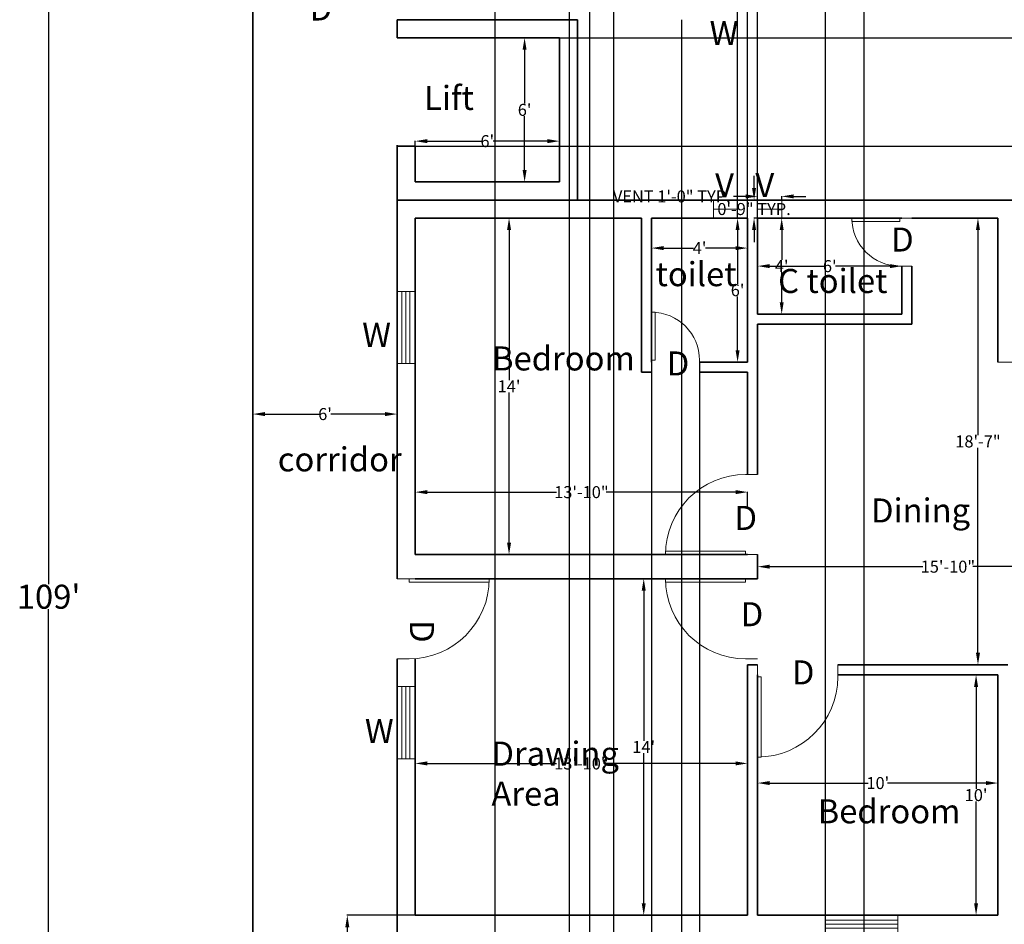
# Model space of a CAD drawing. Units: inches. Extents: x 1936 to 2761, y 1431 to 2889.
# Tile 3 of 6: x 1953 to 2444, y 1999 to 2451. Entities that reach past the tile are written whole.
import ezdxf

# ---------------------------------------------------------------- set-up
doc = ezdxf.new("R2010")
doc.units = ezdxf.units.IN
doc.header["$MEASUREMENT"] = 0
for name, color, linetype, lineweight in [('A-ANNO-DIMS', 172, 'Continuous', 13), ('A-ANNO-TEXT', 50, 'Continuous', 18), ('A-AREA-IDEN', 50, 'Continuous', 18), ('A-FLOR-EVTR', 4, 'Continuous', 35), ('A-FLOR-FIXT', 8, 'Continuous', 18), ('A-GLAZ', 3, 'Continuous', 18), ('A-WALL', 4, 'Continuous', 35), ('doors', 10, 'Continuous', 18)]:
    doc.layers.add(name, color=color, linetype=linetype, lineweight=lineweight)
doc.styles.get("Standard").update_dxf_attribs({"font": 'arial.ttf'})
doc.dimstyles.get("Standard").update_dxf_attribs({"dimtxt": 6, "dimasz": 6, "dimexe": 0.18, "dimexo": 0.0625, "dimgap": 0.09, "dimtad": 0, "dimtih": 1, "dimtoh": 1, "dimdec": 0, "dimzin": 0, "dimdsep": 46, "dimlunit": 3, "dimtxsty": 'Standard', "dimcen": 0.09, "dimadec": 0, "dimazin": 0, "dimtfac": 1, "dimtdec": 0, "dimtofl": 0, "dimtmove": 0, "dimatfit": 3, "dimfxl": 1, "dimtolj": 1, "dimtzin": 0, "dimarcsym": 0})

# ---------------------------------------------------------------- blocks, each defined once
blk = doc.blocks.new('*U4')
for p, q in [((0, 0), (0, 6)), ((24, 0), (24, 6))]:
    blk.add_line(p, q)
blk.add_lwpolyline([(0, 0), (0, -24), (1.75, -24), (1.75, 0)], close=True)
blk.add_arc((0, 0), 24, 270, 0)
blk = doc.blocks.new('*U3')
for p, q in [((0, 0), (0, -6)), ((24, 0), (24, -6))]:
    blk.add_line(p, q)
blk.add_lwpolyline([(0, 0), (0, 24), (1.75, 24), (1.75, 0)], close=True)
blk.add_arc((0, 0), 24, 0, 90)
blk = doc.blocks.new('*U5')
for p, q in [((0, 0), (0, -6)), ((40, 0), (40, -6))]:
    blk.add_line(p, q)
blk.add_lwpolyline([(0, 0), (0, 40), (1.75, 40), (1.75, 0)], close=True)
blk.add_arc((0, 0), 40, 0, 90)
blk = doc.blocks.new('*U2')
for p, q in [((0, 0), (0, 6)), ((40, 0), (40, 6))]:
    blk.add_line(p, q)
blk.add_lwpolyline([(0, 0), (0, -40), (1.75, -40), (1.75, 0)], close=True)
blk.add_arc((0, 0), 40, 270, 360)
blk = doc.blocks.new('*D32')
at = {"layer": 'A-ANNO-DIMS', "color": 0, "lineweight": -2, "transparency": 16777216}
for p, q in [((2150.01, 2207.55), (2150.01, 2214.93)), ((2156.01, 2214.75), (2220.56, 2214.75)), ((2310.01, 2214.75), (2245.45, 2214.75)), ((2316.01, 2207.55), (2316.01, 2214.93))]:
    blk.add_line(p, q, dxfattribs=at)
at = {"layer": 'A-ANNO-DIMS', "color": 0, "transparency": 16777216}
for points in [[(2156.01, 2215.75), (2156.01, 2213.75), (2150.01, 2214.75)], [(2310.01, 2215.75), (2310.01, 2213.75), (2316.01, 2214.75)]]:
    blk.add_solid(points, dxfattribs=at)
at = {"layer": 'Defpoints', "color": 0, "transparency": 16777216}
for p in [(2316.01, 2214.75), (2150.01, 2207.49), (2316.01, 2207.49)]:
    blk.add_point(p, dxfattribs=at)
at = {"layer": 'A-ANNO-DIMS', "color": 0, "transparency": 16777216, "insert": (2233.01, 2214.75), "char_height": 6, "attachment_point": 5}
blk.add_mtext('\\A1;13\'-10"', dxfattribs=at)
blk = doc.blocks.new('*D33')
at = {"layer": 'A-ANNO-DIMS', "color": 0, "lineweight": -2, "transparency": 16777216}
for p, q in [((2196.95, 2351.55), (2197.07, 2351.55)), ((2196.89, 2345.55), (2196.89, 2270.65)), ((2196.89, 2189.55), (2196.89, 2264.45)), ((2196.95, 2183.55), (2197.07, 2183.55))]:
    blk.add_line(p, q, dxfattribs=at)
at = {"layer": 'A-ANNO-DIMS', "color": 0, "transparency": 16777216}
for points in [[(2195.89, 2345.55), (2197.89, 2345.55), (2196.89, 2351.55)], [(2195.89, 2189.55), (2197.89, 2189.55), (2196.89, 2183.55)]]:
    blk.add_solid(points, dxfattribs=at)
at = {"layer": 'Defpoints', "color": 0, "transparency": 16777216}
for p in [(2196.89, 2351.55), (2196.89, 2183.55), (2196.89, 2183.55)]:
    blk.add_point(p, dxfattribs=at)
at = {"layer": 'A-ANNO-DIMS', "color": 0, "transparency": 16777216, "insert": (2196.89, 2267.55), "char_height": 6, "attachment_point": 5}
blk.add_mtext("\\A1;14'", dxfattribs=at)
blk = doc.blocks.new('*D39')
at = {"layer": 'A-ANNO-DIMS', "color": 0, "lineweight": -2, "transparency": 16777216}
for p, q in [((2321.01, 2177.61), (2321.01, 2177.73)), ((2327.01, 2177.55), (2403.56, 2177.55)), ((2505.01, 2177.55), (2428.45, 2177.55)), ((2511.01, 2177.61), (2511.01, 2177.73))]:
    blk.add_line(p, q, dxfattribs=at)
at = {"layer": 'A-ANNO-DIMS', "color": 0, "transparency": 16777216}
for points in [[(2327.01, 2178.55), (2327.01, 2176.55), (2321.01, 2177.55)], [(2505.01, 2178.55), (2505.01, 2176.55), (2511.01, 2177.55)]]:
    blk.add_solid(points, dxfattribs=at)
at = {"layer": 'Defpoints', "color": 0, "transparency": 16777216}
for p in [(2321.01, 2177.55), (2511.01, 2177.55), (2511.01, 2177.55)]:
    blk.add_point(p, dxfattribs=at)
at = {"layer": 'A-ANNO-DIMS', "color": 0, "transparency": 16777216, "insert": (2416.01, 2177.55), "char_height": 6, "attachment_point": 5}
blk.add_mtext('\\A1;15\'-10"', dxfattribs=at)
blk = doc.blocks.new('*D40')
at = {"layer": 'A-ANNO-DIMS', "color": 0, "lineweight": -2, "transparency": 16777216}
for p, q in [((2419.57, 2351.55), (2431.19, 2351.55)), ((2431.01, 2345.55), (2431.01, 2243.2)), ((2431.01, 2134.55), (2431.01, 2236.9)), ((2419.57, 2128.55), (2431.19, 2128.55))]:
    blk.add_line(p, q, dxfattribs=at)
at = {"layer": 'A-ANNO-DIMS', "color": 0, "transparency": 16777216}
for points in [[(2430.01, 2345.55), (2432.01, 2345.55), (2431.01, 2351.55)], [(2430.01, 2134.55), (2432.01, 2134.55), (2431.01, 2128.55)]]:
    blk.add_solid(points, dxfattribs=at)
at = {"layer": 'Defpoints', "color": 0, "transparency": 16777216}
for p in [(2419.51, 2351.55), (2419.51, 2128.55), (2431.01, 2128.55)]:
    blk.add_point(p, dxfattribs=at)
at = {"layer": 'A-ANNO-DIMS', "color": 0, "transparency": 16777216, "insert": (2431.01, 2240.05), "char_height": 6, "attachment_point": 5}
blk.add_mtext('\\A1;18\'-7"', dxfattribs=at)
blk = doc.blocks.new('*D36')
at = {"layer": 'A-ANNO-DIMS', "color": 0, "lineweight": -2, "transparency": 16777216}
for p, q in [((2321.01, 2327.61), (2321.01, 2327.73)), ((2327.01, 2327.55), (2354.14, 2327.55)), ((2387.01, 2327.55), (2359.87, 2327.55)), ((2393.01, 2327.49), (2393.01, 2327.37))]:
    blk.add_line(p, q, dxfattribs=at)
at = {"layer": 'A-ANNO-DIMS', "color": 0, "transparency": 16777216}
for points in [[(2327.01, 2328.55), (2327.01, 2326.55), (2321.01, 2327.55)], [(2387.01, 2328.55), (2387.01, 2326.55), (2393.01, 2327.55)]]:
    blk.add_solid(points, dxfattribs=at)
at = {"layer": 'Defpoints', "color": 0, "transparency": 16777216}
for p in [(2321.01, 2327.55), (2393.01, 2327.55), (2393.01, 2327.55)]:
    blk.add_point(p, dxfattribs=at)
at = {"layer": 'A-ANNO-DIMS', "color": 0, "transparency": 16777216, "insert": (2357.01, 2327.55), "char_height": 6, "attachment_point": 5}
blk.add_mtext("\\A1;6'", dxfattribs=at)
blk = doc.blocks.new('*D37')
at = {"layer": 'A-ANNO-DIMS', "color": 0, "lineweight": -2, "transparency": 16777216}
for p, q in [((2333.07, 2351.55), (2333.19, 2351.55)), ((2333.01, 2345.55), (2333.01, 2330.64)), ((2333.01, 2309.55), (2333.01, 2324.46)), ((2333.07, 2303.55), (2333.19, 2303.55))]:
    blk.add_line(p, q, dxfattribs=at)
at = {"layer": 'A-ANNO-DIMS', "color": 0, "transparency": 16777216}
for points in [[(2332.01, 2345.55), (2334.01, 2345.55), (2333.01, 2351.55)], [(2332.01, 2309.55), (2334.01, 2309.55), (2333.01, 2303.55)]]:
    blk.add_solid(points, dxfattribs=at)
at = {"layer": 'Defpoints', "color": 0, "transparency": 16777216}
for p in [(2333.01, 2351.55), (2333.01, 2303.55), (2333.01, 2303.55)]:
    blk.add_point(p, dxfattribs=at)
at = {"layer": 'A-ANNO-DIMS', "color": 0, "transparency": 16777216, "insert": (2333.01, 2327.55), "char_height": 6, "attachment_point": 5}
blk.add_mtext("\\A1;4'", dxfattribs=at)
blk = doc.blocks.new('*D38')
at = {"layer": 'A-ANNO-DIMS', "color": 0, "lineweight": -2, "transparency": 16777216}
for p, q in [((2306.79, 2351.55), (2311.17, 2351.55)), ((2310.99, 2345.55), (2310.99, 2318.7)), ((2310.99, 2285.55), (2310.99, 2312.4)), ((2306.79, 2279.55), (2311.17, 2279.55))]:
    blk.add_line(p, q, dxfattribs=at)
at = {"layer": 'A-ANNO-DIMS', "color": 0, "transparency": 16777216}
for points in [[(2309.99, 2345.55), (2311.99, 2345.55), (2310.99, 2351.55)], [(2309.99, 2285.55), (2311.99, 2285.55), (2310.99, 2279.55)]]:
    blk.add_solid(points, dxfattribs=at)
at = {"layer": 'Defpoints', "color": 0, "transparency": 16777216}
for p in [(2306.73, 2351.55), (2306.73, 2279.55), (2310.99, 2279.55)]:
    blk.add_point(p, dxfattribs=at)
at = {"layer": 'A-ANNO-DIMS', "color": 0, "transparency": 16777216, "insert": (2310.99, 2315.55), "char_height": 6, "attachment_point": 5}
blk.add_mtext("\\A1;6'", dxfattribs=at)
blk = doc.blocks.new('*D43')
at = {"layer": 'A-ANNO-DIMS', "color": 0, "lineweight": -2, "transparency": 16777216}
for p, q in [((2268.01, 2336.63), (2268.01, 2336.74)), ((2274.01, 2336.56), (2289.03, 2336.56)), ((2310.01, 2336.56), (2294.98, 2336.56)), ((2316.01, 2336.63), (2316.01, 2336.74))]:
    blk.add_line(p, q, dxfattribs=at)
at = {"layer": 'A-ANNO-DIMS', "color": 0, "transparency": 16777216}
for points in [[(2274.01, 2337.56), (2274.01, 2335.56), (2268.01, 2336.56)], [(2310.01, 2337.56), (2310.01, 2335.56), (2316.01, 2336.56)]]:
    blk.add_solid(points, dxfattribs=at)
at = {"layer": 'Defpoints', "color": 0, "transparency": 16777216}
for p in [(2268.01, 2336.56), (2268.01, 2336.56), (2316.01, 2336.56)]:
    blk.add_point(p, dxfattribs=at)
at = {"layer": 'A-ANNO-DIMS', "color": 0, "transparency": 16777216, "insert": (2292.01, 2336.56), "char_height": 6, "attachment_point": 5}
blk.add_mtext("\\A1;4'", dxfattribs=at)
blk = doc.blocks.new('*D44')
at = {"layer": 'A-ANNO-DIMS', "color": 0, "lineweight": -2, "transparency": 16777216}
for p, q in [((2150.01, 2079.41), (2150.01, 2079.53)), ((2156.01, 2079.35), (2220.56, 2079.35)), ((2310.01, 2079.35), (2245.45, 2079.35)), ((2316.01, 2079.41), (2316.01, 2079.53))]:
    blk.add_line(p, q, dxfattribs=at)
at = {"layer": 'A-ANNO-DIMS', "color": 0, "transparency": 16777216}
for points in [[(2156.01, 2080.35), (2156.01, 2078.35), (2150.01, 2079.35)], [(2310.01, 2080.35), (2310.01, 2078.35), (2316.01, 2079.35)]]:
    blk.add_solid(points, dxfattribs=at)
at = {"layer": 'Defpoints', "color": 0, "transparency": 16777216}
for p in [(2150.01, 2079.35), (2316.01, 2079.35), (2316.01, 2079.35)]:
    blk.add_point(p, dxfattribs=at)
at = {"layer": 'A-ANNO-DIMS', "color": 0, "transparency": 16777216, "insert": (2233.01, 2079.35), "char_height": 6, "attachment_point": 5}
blk.add_mtext('\\A1;13\'-10"', dxfattribs=at)
blk = doc.blocks.new('*D45')
at = {"layer": 'A-ANNO-DIMS', "color": 0, "lineweight": -2, "transparency": 16777216}
for p, q in [((2259.65, 2171.55), (2264.3, 2171.55)), ((2264.12, 2165.55), (2264.12, 2090.65)), ((2264.12, 2009.55), (2264.12, 2084.45)), ((2259.65, 2003.55), (2264.3, 2003.55))]:
    blk.add_line(p, q, dxfattribs=at)
at = {"layer": 'A-ANNO-DIMS', "color": 0, "transparency": 16777216}
for points in [[(2263.12, 2165.55), (2265.12, 2165.55), (2264.12, 2171.55)], [(2263.12, 2009.55), (2265.12, 2009.55), (2264.12, 2003.55)]]:
    blk.add_solid(points, dxfattribs=at)
at = {"layer": 'Defpoints', "color": 0, "transparency": 16777216}
for p in [(2259.59, 2171.55), (2259.59, 2003.55), (2264.12, 2003.55)]:
    blk.add_point(p, dxfattribs=at)
at = {"layer": 'A-ANNO-DIMS', "color": 0, "transparency": 16777216, "insert": (2264.12, 2087.55), "char_height": 6, "attachment_point": 5}
blk.add_mtext("\\A1;14'", dxfattribs=at)
blk = doc.blocks.new('*D46')
at = {"layer": 'A-ANNO-DIMS', "color": 0, "lineweight": -2, "transparency": 16777216}
for p, q in [((2321.01, 2063.61), (2321.01, 2069.73)), ((2327.01, 2069.55), (2376.11, 2069.55)), ((2435.01, 2069.55), (2385.91, 2069.55)), ((2441.01, 2063.61), (2441.01, 2069.73))]:
    blk.add_line(p, q, dxfattribs=at)
at = {"layer": 'A-ANNO-DIMS', "color": 0, "transparency": 16777216}
for points in [[(2327.01, 2070.55), (2327.01, 2068.55), (2321.01, 2069.55)], [(2435.01, 2070.55), (2435.01, 2068.55), (2441.01, 2069.55)]]:
    blk.add_solid(points, dxfattribs=at)
at = {"layer": 'Defpoints', "color": 0, "transparency": 16777216}
for p in [(2321.01, 2069.55), (2321.01, 2063.55), (2441.01, 2063.55)]:
    blk.add_point(p, dxfattribs=at)
at = {"layer": 'A-ANNO-DIMS', "color": 0, "transparency": 16777216, "insert": (2381.01, 2069.55), "char_height": 6, "attachment_point": 5}
blk.add_mtext("\\A1;10'", dxfattribs=at)
blk = doc.blocks.new('*D47')
at = {"layer": 'A-ANNO-DIMS', "color": 0, "lineweight": -2, "transparency": 16777216}
for p, q in [((2426.08, 2123.55), (2430.25, 2123.55)), ((2430.07, 2117.55), (2430.07, 2066.7)), ((2430.07, 2009.55), (2430.07, 2060.4)), ((2426.08, 2003.55), (2430.25, 2003.55))]:
    blk.add_line(p, q, dxfattribs=at)
at = {"layer": 'A-ANNO-DIMS', "color": 0, "transparency": 16777216}
for points in [[(2429.07, 2117.55), (2431.07, 2117.55), (2430.07, 2123.55)], [(2429.07, 2009.55), (2431.07, 2009.55), (2430.07, 2003.55)]]:
    blk.add_solid(points, dxfattribs=at)
at = {"layer": 'Defpoints', "color": 0, "transparency": 16777216}
for p in [(2426.02, 2123.55), (2426.02, 2003.55), (2430.07, 2003.55)]:
    blk.add_point(p, dxfattribs=at)
at = {"layer": 'A-ANNO-DIMS', "color": 0, "transparency": 16777216, "insert": (2430.07, 2063.55), "char_height": 6, "attachment_point": 5}
blk.add_mtext("\\A1;10'", dxfattribs=at)
blk = doc.blocks.new('*D54')
at = {"layer": 'A-ANNO-DIMS', "color": 0, "lineweight": -2, "transparency": 16777216}
for p, q in [((2069.01, 2253.77), (2069.01, 2253.89)), ((2075.01, 2253.71), (2102.14, 2253.71)), ((2135.01, 2253.71), (2107.87, 2253.71)), ((2141.01, 2253.77), (2141.01, 2253.89))]:
    blk.add_line(p, q, dxfattribs=at)
at = {"layer": 'A-ANNO-DIMS', "color": 0, "transparency": 16777216}
for points in [[(2075.01, 2254.71), (2075.01, 2252.71), (2069.01, 2253.71)], [(2135.01, 2254.71), (2135.01, 2252.71), (2141.01, 2253.71)]]:
    blk.add_solid(points, dxfattribs=at)
at = {"layer": 'Defpoints', "color": 0, "transparency": 16777216}
for p in [(2069.01, 2253.71), (2141.01, 2253.71), (2141.01, 2253.71)]:
    blk.add_point(p, dxfattribs=at)
at = {"layer": 'A-ANNO-DIMS', "color": 0, "transparency": 16777216, "insert": (2105.01, 2253.71), "char_height": 6, "attachment_point": 5}
blk.add_mtext("\\A1;6'", dxfattribs=at)
blk = doc.blocks.new('*U55')
for p, q in [((-40, 0), (-40, 6)), ((0, 0), (0, 6))]:
    blk.add_line(p, q)
blk.add_lwpolyline([(0, 0), (0, -40), (-1.75, -40), (-1.75, 0)], close=True)
blk.add_arc((0, 0), 40, 180, 270)
blk = doc.blocks.new('*D76')
at = {"layer": 'A-ANNO-DIMS', "color": 0, "lineweight": -2, "transparency": 16777216}
for p, q in [((2068.94, 2816.55), (1966.82, 2816.55)), ((1967, 2810.55), (1967, 2168.77)), ((1967, 1514.55), (1967, 2156.33)), ((2068.94, 1508.55), (1966.82, 1508.55))]:
    blk.add_line(p, q, dxfattribs=at)
at = {"layer": 'A-ANNO-DIMS', "color": 0, "transparency": 16777216}
for points in [[(1966, 2810.55), (1968, 2810.55), (1967, 2816.55)], [(1966, 1514.55), (1968, 1514.55), (1967, 1508.55)]]:
    blk.add_solid(points, dxfattribs=at)
at = {"layer": 'Defpoints', "color": 0, "transparency": 16777216}
for p in [(2069.01, 2816.55), (1967, 1508.55), (2069.01, 1508.55)]:
    blk.add_point(p, dxfattribs=at)
at = {"layer": 'A-ANNO-DIMS', "color": 0, "transparency": 16777216, "insert": (1967, 2162.55), "char_height": 6, "attachment_point": 5}
blk.add_mtext("\\A1;{\\H2x;109'}", dxfattribs=at)
blk = doc.blocks.new('*D77')
at = {"layer": 'A-ANNO-DIMS', "color": 0, "lineweight": -2, "transparency": 16777216}
for p, q in [((2172.87, 2003.55), (2115.94, 2003.55)), ((2116.12, 1997.55), (2116.12, 1961.7)), ((2116.12, 1919.55), (2116.12, 1955.4)), ((2160.94, 1913.55), (2115.94, 1913.55))]:
    blk.add_line(p, q, dxfattribs=at)
at = {"layer": 'A-ANNO-DIMS', "color": 0, "transparency": 16777216}
for points in [[(2115.12, 1997.55), (2117.12, 1997.55), (2116.12, 2003.55)], [(2115.12, 1919.55), (2117.12, 1919.55), (2116.12, 1913.55)]]:
    blk.add_solid(points, dxfattribs=at)
at = {"layer": 'Defpoints', "color": 0, "transparency": 16777216}
for p in [(2172.93, 2003.55), (2116.12, 1913.55), (2161.01, 1913.55)]:
    blk.add_point(p, dxfattribs=at)
at = {"layer": 'A-ANNO-DIMS', "color": 0, "transparency": 16777216, "insert": (2116.12, 1958.55), "char_height": 6, "attachment_point": 5}
blk.add_mtext('\\A1;7\'-6"', dxfattribs=at)
blk = doc.blocks.new('*D78')
at = {"layer": 'A-ANNO-DIMS', "color": 0, "lineweight": -2, "transparency": 16777216}
for p, q in [((2180.03, 2441.55), (2204.82, 2441.55)), ((2204.64, 2435.55), (2204.64, 2408.7)), ((2204.64, 2375.55), (2204.64, 2402.4)), ((2172.39, 2369.55), (2204.82, 2369.55))]:
    blk.add_line(p, q, dxfattribs=at)
at = {"layer": 'A-ANNO-DIMS', "color": 0, "transparency": 16777216}
for points in [[(2203.64, 2435.55), (2205.64, 2435.55), (2204.64, 2441.55)], [(2203.64, 2375.55), (2205.64, 2375.55), (2204.64, 2369.55)]]:
    blk.add_solid(points, dxfattribs=at)
at = {"layer": 'Defpoints', "color": 0, "transparency": 16777216}
for p in [(2179.96, 2441.55), (2172.33, 2369.55), (2204.64, 2369.55)]:
    blk.add_point(p, dxfattribs=at)
at = {"layer": 'A-ANNO-DIMS', "color": 0, "transparency": 16777216, "insert": (2204.64, 2405.55), "char_height": 6, "attachment_point": 5}
blk.add_mtext("\\A1;6'", dxfattribs=at)
blk = doc.blocks.new('*D79')
at = {"layer": 'A-ANNO-DIMS', "color": 0, "lineweight": -2, "transparency": 16777216}
for p, q in [((2150.01, 2378.56), (2150.01, 2390.12)), ((2156.01, 2389.94), (2183.14, 2389.94)), ((2216.01, 2389.94), (2188.87, 2389.94)), ((2222.01, 2378.56), (2222.01, 2390.12))]:
    blk.add_line(p, q, dxfattribs=at)
at = {"layer": 'A-ANNO-DIMS', "color": 0, "transparency": 16777216}
for points in [[(2156.01, 2390.94), (2156.01, 2388.94), (2150.01, 2389.94)], [(2216.01, 2390.94), (2216.01, 2388.94), (2222.01, 2389.94)]]:
    blk.add_solid(points, dxfattribs=at)
at = {"layer": 'Defpoints', "color": 0, "transparency": 16777216}
for p in [(2222.01, 2389.94), (2150.01, 2378.5), (2222.01, 2378.5)]:
    blk.add_point(p, dxfattribs=at)
at = {"layer": 'A-ANNO-DIMS', "color": 0, "transparency": 16777216, "insert": (2186.01, 2389.94), "char_height": 6, "attachment_point": 5}
blk.add_mtext("\\A1;6'", dxfattribs=at)
blk = doc.blocks.new('WIN-36')
for p, q in [((0, 9), (0, 0)), ((36, 6.5), (0, 6.5)), ((36, 9), (36, 0)), ((36, 4.5), (0, 4.5)), ((36, 2.5), (0, 2.5))]:
    blk.add_line(p, q)
blk = doc.blocks.new('VENT-12')
for p, q in [((0, 0), (0, 9)), ((12, 0), (12, 9)), ((0, 4.5), (12, 4.5))]:
    blk.add_line(p, q)
blk = doc.blocks.new('COUNTER-KITCHEN-U')
for p, q in [((41, 36), (41, 0)), ((41, 36), (135, 36)), ((135, 36), (135, 0)), ((0, 0), (41, 0)), ((135, 0), (171, 0))]:
    blk.add_line(p, q)
blk = doc.blocks.new('*D89')
at = {"layer": 'A-ANNO-DIMS', "color": 0, "lineweight": -2, "transparency": 16777216}
for p, q in [((2315.01, 2362.35), (2309.01, 2362.35)), ((2321.01, 2360.61), (2321.01, 2362.53)), ((2333.01, 2360.61), (2333.01, 2362.53)), ((2339.01, 2362.35), (2345.01, 2362.35))]:
    blk.add_line(p, q, dxfattribs=at)
at = {"layer": 'A-ANNO-DIMS', "color": 0, "transparency": 16777216}
for points in [[(2315.01, 2363.35), (2315.01, 2361.35), (2321.01, 2362.35)], [(2339.01, 2363.35), (2339.01, 2361.35), (2333.01, 2362.35)]]:
    blk.add_solid(points, dxfattribs=at)
at = {"layer": 'Defpoints', "color": 0, "transparency": 16777216}
for p in [(2321.01, 2362.35), (2321.01, 2360.55), (2333.01, 2360.55)]:
    blk.add_point(p, dxfattribs=at)
at = {"layer": 'A-ANNO-DIMS', "color": 0, "transparency": 16777216, "insert": (2278.13, 2362.35), "char_height": 6, "attachment_point": 5}
blk.add_mtext('\\A1;VENT 1\'-0" TYP.', dxfattribs=at)
blk = doc.blocks.new('*D90')
at = {"layer": 'A-ANNO-DIMS', "color": 0, "lineweight": -2, "transparency": 16777216}
for p, q in [((2319.21, 2366.55), (2319.21, 2372.55)), ((2320.94, 2360.55), (2319.03, 2360.55)), ((2320.94, 2351.55), (2319.03, 2351.55)), ((2319.21, 2345.55), (2319.21, 2339.55))]:
    blk.add_line(p, q, dxfattribs=at)
at = {"layer": 'A-ANNO-DIMS', "color": 0, "transparency": 16777216}
for points in [[(2318.21, 2366.55), (2320.21, 2366.55), (2319.21, 2360.55)], [(2318.21, 2345.55), (2320.21, 2345.55), (2319.21, 2351.55)]]:
    blk.add_solid(points, dxfattribs=at)
at = {"layer": 'Defpoints', "color": 0, "transparency": 16777216}
for p in [(2321.01, 2360.55), (2319.21, 2351.55), (2321.01, 2351.55)]:
    blk.add_point(p, dxfattribs=at)
at = {"layer": 'A-ANNO-DIMS', "color": 0, "transparency": 16777216, "insert": (2319.21, 2356.05), "char_height": 6, "attachment_point": 5}
blk.add_mtext('\\A1;0\'-9" TYP.', dxfattribs=at)
blk = doc.blocks.new('*D99')
at = {"layer": 'A-ANNO-DIMS', "color": 0, "lineweight": -2, "transparency": 16777216}
for p, q in [((2021.01, 2816.61), (2021.01, 2885.73)), ((2027.01, 2885.55), (2334.61, 2885.55)), ((2663.01, 2885.55), (2355.4, 2885.55)), ((2669.01, 2360.61), (2669.01, 2885.73))]:
    blk.add_line(p, q, dxfattribs=at)
at = {"layer": 'A-ANNO-DIMS', "color": 0, "transparency": 16777216}
for points in [[(2027.01, 2886.55), (2027.01, 2884.55), (2021.01, 2885.55)], [(2663.01, 2886.55), (2663.01, 2884.55), (2669.01, 2885.55)]]:
    blk.add_solid(points, dxfattribs=at)
at = {"layer": 'Defpoints', "color": 0, "transparency": 16777216}
for p in [(2669.01, 2885.55), (2021.01, 2816.55), (2669.01, 2360.55)]:
    blk.add_point(p, dxfattribs=at)
at = {"layer": 'A-ANNO-DIMS', "color": 0, "transparency": 16777216, "insert": (2345.01, 2885.55), "char_height": 6, "attachment_point": 5}
blk.add_mtext('\\A1;54\'-0"', dxfattribs=at)
blk = doc.blocks.new('*D104')
at = {"layer": 'A-ANNO-DIMS', "color": 0, "lineweight": -2, "transparency": 16777216}
for p, q in [((2190.01, 1922.61), (2190.01, 2885.73)), ((2196.01, 2885.55), (2262.35, 2885.55)), ((2348.92, 2885.55), (2282.58, 2885.55)), ((2354.92, 1922.61), (2354.92, 2885.73))]:
    blk.add_line(p, q, dxfattribs=at)
at = {"layer": 'A-ANNO-DIMS', "color": 0, "transparency": 16777216}
for points in [[(2196.01, 2886.55), (2196.01, 2884.55), (2190.01, 2885.55)], [(2348.92, 2886.55), (2348.92, 2884.55), (2354.92, 2885.55)]]:
    blk.add_solid(points, dxfattribs=at)
at = {"layer": 'Defpoints', "color": 0, "transparency": 16777216}
for p in [(2354.92, 2885.55), (2190.01, 1922.55), (2354.92, 1922.55)]:
    blk.add_point(p, dxfattribs=at)
at = {"layer": 'A-ANNO-DIMS', "color": 0, "transparency": 16777216, "insert": (2272.46, 2885.55), "char_height": 6, "attachment_point": 5}
blk.add_mtext('\\A1;13\'-9"', dxfattribs=at)
blk = doc.blocks.new('*D107')
at = {"layer": 'A-ANNO-DIMS', "color": 0, "lineweight": -2, "transparency": 16777216}
for p, q in [((2221.14, 2885.55), (2215.14, 2885.55)), ((2227.14, 1922.61), (2227.14, 2885.73)), ((2237.14, 1922.61), (2237.14, 2885.73)), ((2243.14, 2885.55), (2249.14, 2885.55))]:
    blk.add_line(p, q, dxfattribs=at)
at = {"layer": 'A-ANNO-DIMS', "color": 0, "transparency": 16777216}
for points in [[(2221.14, 2886.55), (2221.14, 2884.55), (2227.14, 2885.55)], [(2243.14, 2886.55), (2243.14, 2884.55), (2237.14, 2885.55)]]:
    blk.add_solid(points, dxfattribs=at)
at = {"layer": 'Defpoints', "color": 0, "transparency": 16777216}
for p in [(2237.14, 2885.55), (2227.14, 1922.55), (2237.14, 1922.55)]:
    blk.add_point(p, dxfattribs=at)
at = {"layer": 'A-ANNO-DIMS', "color": 0, "transparency": 16777216, "insert": (2259.54, 2885.55), "char_height": 6, "attachment_point": 5}
blk.add_mtext('\\A1;0\'-10"', dxfattribs=at)
blk = doc.blocks.new('*D108')
at = {"layer": 'A-ANNO-DIMS', "color": 0, "lineweight": -2, "transparency": 16777216}
for p, q in [((2141.07, 2441.55), (2738.19, 2441.55)), ((2738.01, 2435.55), (2738.01, 2417.65)), ((2738.01, 2393.45), (2738.01, 2411.34)), ((2141.07, 2387.45), (2738.19, 2387.45))]:
    blk.add_line(p, q, dxfattribs=at)
at = {"layer": 'A-ANNO-DIMS', "color": 0, "transparency": 16777216}
for points in [[(2737.01, 2435.55), (2739.01, 2435.55), (2738.01, 2441.55)], [(2737.01, 2393.45), (2739.01, 2393.45), (2738.01, 2387.45)]]:
    blk.add_solid(points, dxfattribs=at)
at = {"layer": 'Defpoints', "color": 0, "transparency": 16777216}
for p in [(2141.01, 2441.55), (2738.01, 2441.55), (2141.01, 2387.45)]:
    blk.add_point(p, dxfattribs=at)
at = {"layer": 'A-ANNO-DIMS', "color": 0, "transparency": 16777216, "insert": (2738.01, 2414.5), "char_height": 6, "attachment_point": 5}
blk.add_mtext('\\A1;4\'-6"', dxfattribs=at)
blk = doc.blocks.new('*D110')
at = {"layer": 'A-ANNO-DIMS', "color": 0, "lineweight": -2, "transparency": 16777216}
for p, q in [((2268.006183, 2279.486911), (2268.006183, 1439.369411)), ((2292.006183, 2279.486911), (2292.006183, 1439.369411)), ((2262.006183, 1439.549411), (2256.006183, 1439.549411)), ((2298.006183, 1439.549411), (2304.006183, 1439.549411))]:
    blk.add_line(p, q, dxfattribs=at)
at = {"layer": 'A-ANNO-DIMS', "color": 0, "transparency": 16777216}
for points in [[(2262.006183, 1440.549411), (2262.006183, 1438.549411), (2268.006183, 1439.549411)], [(2298.006183, 1440.549411), (2298.006183, 1438.549411), (2292.006183, 1439.549411)]]:
    blk.add_solid(points, dxfattribs=at)
at = {"layer": 'Defpoints', "color": 0, "transparency": 16777216}
for p in [(2268.006183, 2279.549411), (2292.006183, 2279.549411), (2292.006183, 1439.549411)]:
    blk.add_point(p, dxfattribs=at)
at = {"layer": 'A-ANNO-DIMS', "color": 0, "transparency": 16777216, "insert": (2280.006183, 1439.549411), "char_height": 6, "attachment_point": 5}
blk.add_mtext('\\A1;2\'-0"', dxfattribs=at)
blk = doc.blocks.new('*D111')
at = {"layer": 'A-ANNO-DIMS', "color": 0, "lineweight": -2, "transparency": 16777216}
for p, q in [((2310.01, 2885.55), (2304.01, 2885.55)), ((2316.01, 2351.61), (2316.01, 2885.73)), ((2321.01, 2351.61), (2321.01, 2885.73)), ((2327.01, 2885.55), (2333.01, 2885.55))]:
    blk.add_line(p, q, dxfattribs=at)
at = {"layer": 'A-ANNO-DIMS', "color": 0, "transparency": 16777216}
for points in [[(2310.01, 2886.55), (2310.01, 2884.55), (2316.01, 2885.55)], [(2327.01, 2886.55), (2327.01, 2884.55), (2321.01, 2885.55)]]:
    blk.add_solid(points, dxfattribs=at)
at = {"layer": 'Defpoints', "color": 0, "transparency": 16777216}
for p in [(2321.01, 2885.55), (2316.01, 2351.55), (2321.01, 2351.55)]:
    blk.add_point(p, dxfattribs=at)
at = {"layer": 'A-ANNO-DIMS', "color": 0, "transparency": 16777216, "insert": (2341.07, 2885.55), "char_height": 6, "attachment_point": 5}
blk.add_mtext('\\A1;0\'-5"', dxfattribs=at)
blk = doc.blocks.new('*D112')
at = {"layer": 'A-ANNO-DIMS', "color": 0, "lineweight": -2, "transparency": 16777216}
for p, q in [((2374.01, 2459.49), (2374.01, 1439.37)), ((2458.21, 2459.49), (2458.21, 1439.37)), ((2380.01, 1439.55), (2408.07, 1439.55)), ((2452.21, 1439.55), (2424.15, 1439.55))]:
    blk.add_line(p, q, dxfattribs=at)
at = {"layer": 'A-ANNO-DIMS', "color": 0, "transparency": 16777216}
for points in [[(2380.01, 1440.55), (2380.01, 1438.55), (2374.01, 1439.55)], [(2452.21, 1440.55), (2452.21, 1438.55), (2458.21, 1439.55)]]:
    blk.add_solid(points, dxfattribs=at)
at = {"layer": 'Defpoints', "color": 0, "transparency": 16777216}
for p in [(2374.01, 2459.55), (2458.21, 2459.55), (2458.21, 1439.55)]:
    blk.add_point(p, dxfattribs=at)
at = {"layer": 'A-ANNO-DIMS', "color": 0, "transparency": 16777216, "insert": (2416.11, 1439.55), "char_height": 6, "attachment_point": 5}
blk.add_mtext('\\A1;7\'-0"', dxfattribs=at)
blk = doc.blocks.new('*D114')
at = {"layer": 'A-ANNO-DIMS', "color": 0, "lineweight": -2, "transparency": 16777216}
for p, q in [((2305.01, 2885.55), (2299.01, 2885.55)), ((2311.01, 2351.61), (2311.01, 2885.73)), ((2316.01, 2351.61), (2316.01, 2885.73)), ((2322.01, 2885.55), (2328.01, 2885.55))]:
    blk.add_line(p, q, dxfattribs=at)
at = {"layer": 'A-ANNO-DIMS', "color": 0, "transparency": 16777216}
for points in [[(2305.01, 2886.55), (2305.01, 2884.55), (2311.01, 2885.55)], [(2322.01, 2886.55), (2322.01, 2884.55), (2316.01, 2885.55)]]:
    blk.add_solid(points, dxfattribs=at)
at = {"layer": 'Defpoints', "color": 0, "transparency": 16777216}
for p in [(2316.01, 2885.55), (2311.01, 2351.55), (2316.01, 2351.55)]:
    blk.add_point(p, dxfattribs=at)
at = {"layer": 'A-ANNO-DIMS', "color": 0, "transparency": 16777216, "insert": (2336.07, 2885.55), "char_height": 6, "attachment_point": 5}
blk.add_mtext('\\A1;0\'-5"', dxfattribs=at)
blk = doc.blocks.new('*D120')
at = {"layer": 'A-ANNO-DIMS', "color": 0, "lineweight": -2, "transparency": 16777216}
for p, q in [((2249.01, 2459.49), (2249.01, 1439.37)), ((2282.92, 2450.49), (2282.92, 1439.37)), ((2255.01, 1439.55), (2255.52, 1439.55)), ((2276.92, 1439.55), (2276.41, 1439.55))]:
    blk.add_line(p, q, dxfattribs=at)
at = {"layer": 'A-ANNO-DIMS', "color": 0, "transparency": 16777216}
for points in [[(2255.01, 1440.55), (2255.01, 1438.55), (2249.01, 1439.55)], [(2276.92, 1440.55), (2276.92, 1438.55), (2282.92, 1439.55)]]:
    blk.add_solid(points, dxfattribs=at)
at = {"layer": 'Defpoints', "color": 0, "transparency": 16777216}
for p in [(2249.01, 2459.55), (2282.92, 2450.55), (2282.92, 1439.55)]:
    blk.add_point(p, dxfattribs=at)
at = {"layer": 'A-ANNO-DIMS', "color": 0, "transparency": 16777216, "insert": (2265.96, 1439.55), "char_height": 6, "attachment_point": 5}
blk.add_mtext('\\A1;2\'-10"', dxfattribs=at)

msp = doc.modelspace()

# ---------------------------------------------------------------- linework, layer by layer
at = {"layer": 'A-FLOR-EVTR'}
for p, q in [((2141.01, 2450.55), (2231.01, 2450.55)), ((2141.01, 2441.55), (2141.01, 2450.55)), ((2231.01, 2450.55), (2231.01, 2360.55)), ((2150.01, 2441.55), (2141.01, 2441.55)), ((2150.01, 2441.55), (2222.01, 2441.55)), ((2222.01, 2441.55), (2222.01, 2369.55)), ((2141.01, 2360.55), (2141.01, 2387.96)), ((2150.01, 2387.45), (2141.01, 2387.45)), ((2150.01, 2369.55), (2150.01, 2387.45)), ((2222.01, 2369.55), (2150.01, 2369.55)), ((2231.01, 2360.55), (2141.01, 2360.55))]:
    msp.add_line(p, q, dxfattribs=at)
at = {"layer": 'A-WALL'}
for p, q in [((2069.01, 1867.87), (2069.01, 2639.55)), ((2141.01, 2360.55), (2621.01, 2360.55)), ((2141.01, 2171.55), (2141.01, 2360.55)), ((2150.01, 2183.55), (2150.01, 2351.55)), ((2150.01, 2351.55), (2263.01, 2351.55)), ((2263.01, 2274.55), (2263.01, 2351.55)), ((2268.01, 2279.55), (2268.01, 2351.55)), ((2268.01, 2351.55), (2316.01, 2351.55)), ((2316.01, 2279.55), (2316.01, 2351.55)), ((2321.01, 2303.55), (2321.01, 2351.55)), ((2321.01, 2351.55), (2393.01, 2351.55)), ((2398.01, 2351.55), (2441.01, 2351.55)), ((2441.01, 2351.55), (2441.01, 2279.55)), ((2393.01, 2303.55), (2393.01, 2327.55)), ((2398.01, 2298.55), (2398.01, 2327.55)), ((2321.01, 2303.55), (2393.01, 2303.55)), ((2321.01, 2223.55), (2321.01, 2298.55)), ((2321.01, 2298.55), (2398.01, 2298.55)), ((2292.01, 2279.55), (2316.01, 2279.55)), ((2263.01, 2274.55), (2268.01, 2274.55)), ((2292.01, 2274.55), (2316.01, 2274.55)), ((2316.01, 2223.55), (2316.01, 2274.55)), ((2150.01, 2183.55), (2316.01, 2183.55)), ((2321.01, 2171.55), (2321.01, 2183.55)), ((2321.01, 2171.55), (2150.01, 2171.55)), ((2141.01, 1994.55), (2141.01, 2131.55)), ((2150.01, 2003.55), (2150.01, 2131.66)), ((2321.01, 2128.55), (2316.01, 2128.55)), ((2316.01, 2003.55), (2316.01, 2128.55)), ((2446.01, 2128.55), (2361.01, 2128.55)), ((2321.01, 2003.55), (2321.01, 2123.55)), ((2441.01, 2123.55), (2361.01, 2123.55)), ((2441.01, 2123.55), (2441.01, 2003.55)), ((2316.01, 2003.55), (2150.01, 2003.55)), ((2441.01, 2003.55), (2321.01, 2003.55))]:
    msp.add_line(p, q, dxfattribs=at)
at = {"layer": 'doors'}
for p, q in [((2398.01, 2351.55), (2393.01, 2351.55)), ((2398.01, 2327.55), (2393.01, 2327.55)), ((2268.01, 2279.55), (2268.01, 2274.55)), ((2292.01, 2279.55), (2292.01, 2274.55)), ((2316.01, 2223.55), (2321.01, 2223.55)), ((2316.01, 2183.55), (2321.01, 2183.55)), ((2150.01, 2171.55), (2141.01, 2171.55)), ((2321.01, 2128.55), (2321.01, 2123.55)), ((2361.01, 2128.55), (2361.01, 2123.55))]:
    msp.add_line(p, q, dxfattribs=at)

# ---------------------------------------------------------------- block references
at = {"layer": 'A-FLOR-FIXT'}
msp.add_blockref('COUNTER-KITCHEN-U', (2441.01, 2279.55), dxfattribs=at)
at = {"layer": 'A-GLAZ'}
for name, p in [('VENT-12', (2299.01, 2351.55)), ('WIN-36', (2354.92, 1994.55))]:
    msp.add_blockref(name, p, dxfattribs=at)
for name, p, rotation in [('VENT-12', (2333.01, 2360.55), 180), ('WIN-36', (2140.9, 2314.89), 269.9999999999969), ('WIN-36', (2140.9, 2117.66), 269.9999999999969)]:
    msp.add_blockref(name, p, dxfattribs=dict(at, rotation=rotation))
at = {"layer": 'doors'}
for name, p, rotation in [('*U4', (2392.01, 2351.55), 270), ('*U5', (2315.01, 2183.55), 90), ('*U55', (2147.01, 2171.55), 90)]:
    msp.add_blockref(name, p, dxfattribs=dict(at, rotation=rotation))
for name, p in [('*U3', (2268.01, 2280.55)), ('*U2', (2321.01, 2122.55))]:
    msp.add_blockref(name, p, dxfattribs=at)
at = {"layer": 'doors', "xscale": -1, "rotation": 90}
msp.add_blockref('*U5', (2315.01, 2171.55), dxfattribs=at)

# ---------------------------------------------------------------- texts
at = {"layer": 'A-ANNO-TEXT', "char_height": 12, "attachment_point": 1}
for s, width, heights, insert in [('D', 28.2371, [0.2], (2097.33, 2462.15)), ('W', 7.8209, [0.2], (2297.01, 2449.85)), ('V', 13.1151, [0], (2299.76, 2373.91)), ('V', 13.1151, [0], (2319.86, 2373.99)), ('D', 28.2371, [0.2], (2387.67, 2346.82)), ('W', 7.8209, [0.2], (2123.56, 2299.26)), ('D', 28.2371, [0.2], (2275.61, 2284.98)), ('D', 28.2371, [0.2], (2309.43, 2207.85)), ('D', 28.2371, [0.2], (2312.54, 2159.8)), ('D', 28.2371, [0.2], (2338.1, 2130.78)), ('W', 7.8209, [0.2], (2124.91, 2101.48))]:
    msp.add_mtext_dynamic_manual_height_columns(s, width=width, gutter_width=1, heights=heights, dxfattribs=dict(at, insert=insert))
at = {"layer": 'A-ANNO-TEXT', "insert": (2159.4, 2150.88), "char_height": 12, "attachment_point": 1, "rotation": 270}
msp.add_mtext_dynamic_manual_height_columns('D', width=28.2371, gutter_width=1, heights=[0.2], dxfattribs=at)
at = {"layer": 'A-AREA-IDEN', "char_height": 12, "attachment_point": 1}
for s, width, insert in [('Lift', 28.1224, (2154.46, 2417.52)), ('toilet', 55.7076, (2270.01, 2329.55)), ('C toilet', 55.7076, (2331.23, 2326.15)), ('Bedroom', 55.7076, (2188.37, 2287.48)), ('corridor', 14.5111, (2081.38, 2237.11)), ('Dining', 55.7076, (2377.61, 2211.6)), ('Drawing Area', 55.7076, (2188.07, 2090.22)), ('Bedroom', 55.7076, (2350.96, 2061.45))]:
    msp.add_mtext_dynamic_manual_height_columns(s, width=width, gutter_width=1, heights=[0], dxfattribs=dict(at, insert=insert))

# ---------------------------------------------------------------- dimensions: what is measured, and where the dimension line sits
at = {"layer": 'A-ANNO-DIMS'}
for base, p1, p2, override, picture, middle in [((2669.01, 2885.55), (2021.01, 2816.55), (2669.01, 2360.55), {"dimdec": 1, "dimlfac": 1, "dimrnd": 0, "dimzin": 1, "dimdsep": 46, "dimlunit": 4, "dimfrac": 2}, '*D99', (2345.01, 2885.55)), ((2354.92, 2885.55), (2190.01, 1922.55), (2354.92, 1922.55), {"dimdec": 1, "dimlfac": 1, "dimrnd": 0, "dimzin": 1, "dimdsep": 46, "dimlunit": 4, "dimfrac": 2}, '*D104', (2272.46, 2885.55)), ((2237.14, 2885.55), (2227.14, 1922.55), (2237.14, 1922.55), {"dimdec": 1, "dimlfac": 1, "dimrnd": 0, "dimzin": 1, "dimdsep": 46, "dimlunit": 4, "dimfrac": 2}, '*D107', (2259.54, 2885.55)), ((2316.01, 2885.55), (2311.01, 2351.55), (2316.01, 2351.55), {"dimdec": 1, "dimlfac": 1, "dimrnd": 0, "dimzin": 1, "dimdsep": 46, "dimlunit": 4, "dimfrac": 2}, '*D114', (2336.07, 2885.55)), ((2321.01, 2885.55), (2316.01, 2351.55), (2321.01, 2351.55), {"dimdec": 1, "dimlfac": 1, "dimrnd": 0, "dimzin": 1, "dimdsep": 46, "dimlunit": 4, "dimfrac": 2}, '*D111', (2341.07, 2885.55)), ((2282.92, 1439.55), (2249.01, 2459.55), (2282.92, 2450.55), {"dimdec": 1, "dimlfac": 1, "dimrnd": 0, "dimzin": 1, "dimdsep": 46, "dimlunit": 4, "dimfrac": 2}, '*D120', (2265.96, 1439.55)), ((2458.21, 1439.55), (2374.01, 2459.55), (2458.21, 2459.55), {"dimdec": 1, "dimlfac": 1, "dimrnd": 0, "dimzin": 1, "dimdsep": 46, "dimlunit": 4, "dimfrac": 2}, '*D112', (2416.11, 1439.55)), ((2222.01, 2389.94), (2150.01, 2378.5), (2222.01, 2378.5), {"dimclrd": 0, "dimclre": 0, "dimclrt": 0}, '*D79', (2186.01, 2389.94)), ((2268.01, 2336.56), (2316.01, 2336.56), (2268.01, 2336.56), {"dimclrd": 0, "dimclre": 0, "dimclrt": 0}, '*D43', (2292.01, 2336.56)), ((2393.01, 2327.55), (2321.01, 2327.55), (2393.01, 2327.55), {"dimclrd": 0, "dimclre": 0, "dimclrt": 0}, '*D36', (2357.01, 2327.55)), ((2292.01, 1439.55), (2268.01, 2279.55), (2292.01, 2279.55), {"dimdec": 1, "dimlfac": 1, "dimrnd": 0, "dimzin": 1, "dimdsep": 46, "dimlunit": 4, "dimfrac": 2}, '*D110', (2280.01, 1439.55)), ((2141.01, 2253.71), (2069.01, 2253.71), (2141.01, 2253.71), {"dimclrd": 0, "dimclre": 0, "dimclrt": 0}, '*D54', (2105.01, 2253.71)), ((2316.01, 2214.75), (2150.01, 2207.49), (2316.01, 2207.49), {"dimclrd": 0, "dimclre": 0, "dimclrt": 0}, '*D32', (2233.01, 2214.75)), ((2511.01, 2177.55), (2321.01, 2177.55), (2511.01, 2177.55), {"dimclrd": 0, "dimclre": 0, "dimclrt": 0}, '*D39', (2416.01, 2177.55)), ((2316.01, 2079.35), (2150.01, 2079.35), (2316.01, 2079.35), {"dimclrd": 0, "dimclre": 0, "dimclrt": 0}, '*D44', (2233.01, 2079.35)), ((2321.01, 2069.55), (2441.01, 2063.55), (2321.01, 2063.55), {"dimclrd": 0, "dimclre": 0, "dimclrt": 0}, '*D46', (2381.01, 2069.55))]:
    dim = msp.add_linear_dim(base=base, p1=p1, p2=p2, dimstyle='Standard', override=override, dxfattribs=at)
    dim.commit()
    dim.dimension.update_dxf_attribs({"geometry": picture, "text_midpoint": middle})
for base, p1, p2, angle, text, override, picture, middle in [((1967, 1508.55), (2069.01, 2816.55), (2069.01, 1508.55), 90, '{\\H2x;<>}', {"dimclrd": 0, "dimclre": 0, "dimclrt": 0}, '*D76', (1967, 2162.55)), ((2321.01, 2362.35), (2333.01, 2360.55), (2321.01, 2360.55), 180, 'VENT <> TYP.', {"dimdec": 1, "dimlfac": 1, "dimrnd": 0, "dimzin": 1, "dimdsep": 46, "dimlunit": 4, "dimfrac": 2}, '*D89', (2278.13, 2362.35)), ((2319.21, 2351.55), (2321.01, 2360.55), (2321.01, 2351.55), 270, '<> TYP.', {"dimdec": 1, "dimlfac": 1, "dimrnd": 0, "dimzin": 1, "dimdsep": 46, "dimlunit": 4, "dimfrac": 2}, '*D90', (2319.21, 2356.05))]:
    dim = msp.add_linear_dim(base=base, p1=p1, p2=p2, angle=angle, text=text, dimstyle='Standard', override=override, dxfattribs=at)
    dim.commit()
    dim.dimension.update_dxf_attribs({"geometry": picture, "text_midpoint": middle})
for base, p1, p2, override, picture, middle in [((2738.01, 2441.55), (2141.01, 2387.45), (2141.01, 2441.55), {"dimdec": 1, "dimlfac": 1, "dimrnd": 0, "dimzin": 1, "dimdsep": 46, "dimlunit": 4, "dimfrac": 2}, '*D108', (2738.01, 2414.5)), ((2204.64, 2369.55), (2179.96, 2441.55), (2172.33, 2369.55), {"dimclrd": 0, "dimclre": 0, "dimclrt": 0}, '*D78', (2204.64, 2405.55)), ((2196.89, 2183.55), (2196.89, 2351.55), (2196.89, 2183.55), {"dimclrd": 0, "dimclre": 0, "dimclrt": 0}, '*D33', (2196.89, 2267.55)), ((2310.99, 2279.55), (2306.73, 2351.55), (2306.73, 2279.55), {"dimclrd": 0, "dimclre": 0, "dimclrt": 0}, '*D38', (2310.99, 2315.55)), ((2333.01, 2303.55), (2333.01, 2351.55), (2333.01, 2303.55), {"dimclrd": 0, "dimclre": 0, "dimclrt": 0}, '*D37', (2333.01, 2327.55)), ((2431.01, 2128.55), (2419.51, 2351.55), (2419.51, 2128.55), {"dimclrd": 0, "dimclre": 0, "dimclrt": 0}, '*D40', (2431.01, 2240.05)), ((2264.12, 2003.55), (2259.59, 2171.55), (2259.59, 2003.55), {"dimclrd": 0, "dimclre": 0, "dimclrt": 0}, '*D45', (2264.12, 2087.55)), ((2430.07, 2003.55), (2426.02, 2123.55), (2426.02, 2003.55), {"dimclrd": 0, "dimclre": 0, "dimclrt": 0}, '*D47', (2430.07, 2063.55)), ((2116.12, 1913.55), (2172.93, 2003.55), (2161.01, 1913.55), {"dimclrd": 0, "dimclre": 0, "dimclrt": 0}, '*D77', (2116.12, 1958.55))]:
    dim = msp.add_linear_dim(base=base, p1=p1, p2=p2, angle=90, dimstyle='Standard', override=override, dxfattribs=at)
    dim.commit()
    dim.dimension.update_dxf_attribs({"geometry": picture, "text_midpoint": middle})

doc.saveas('drawing.dxf')
